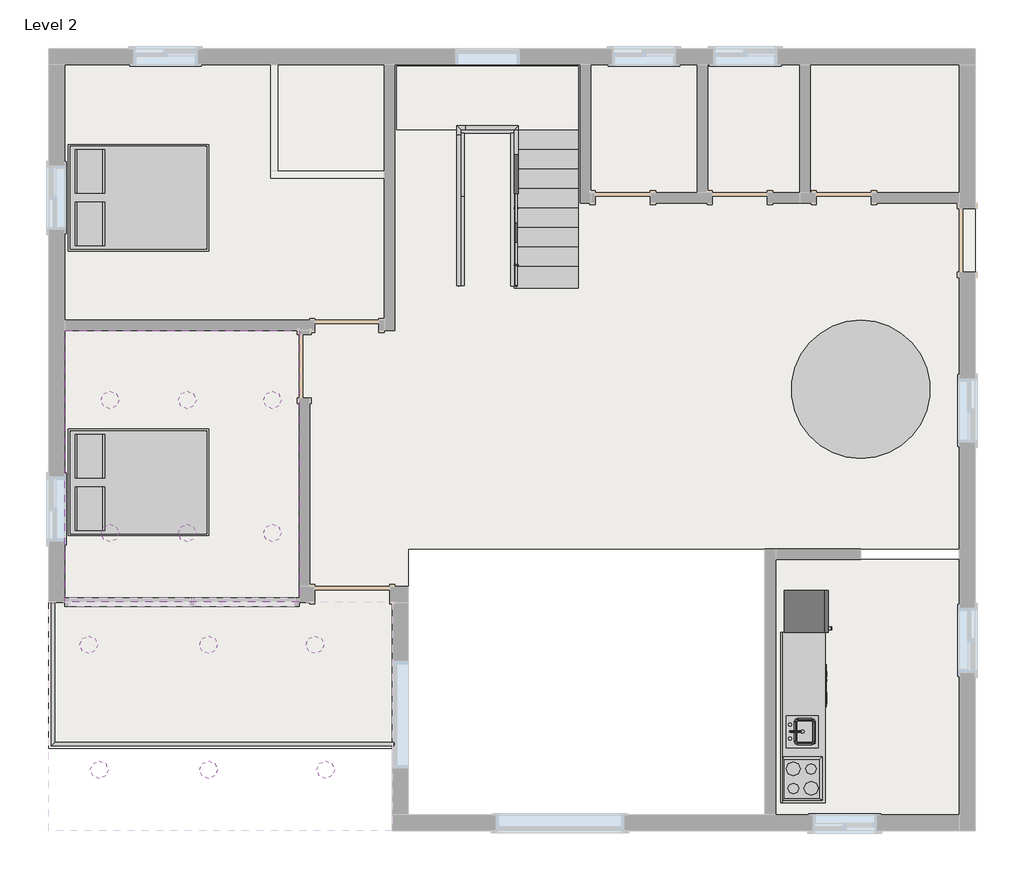
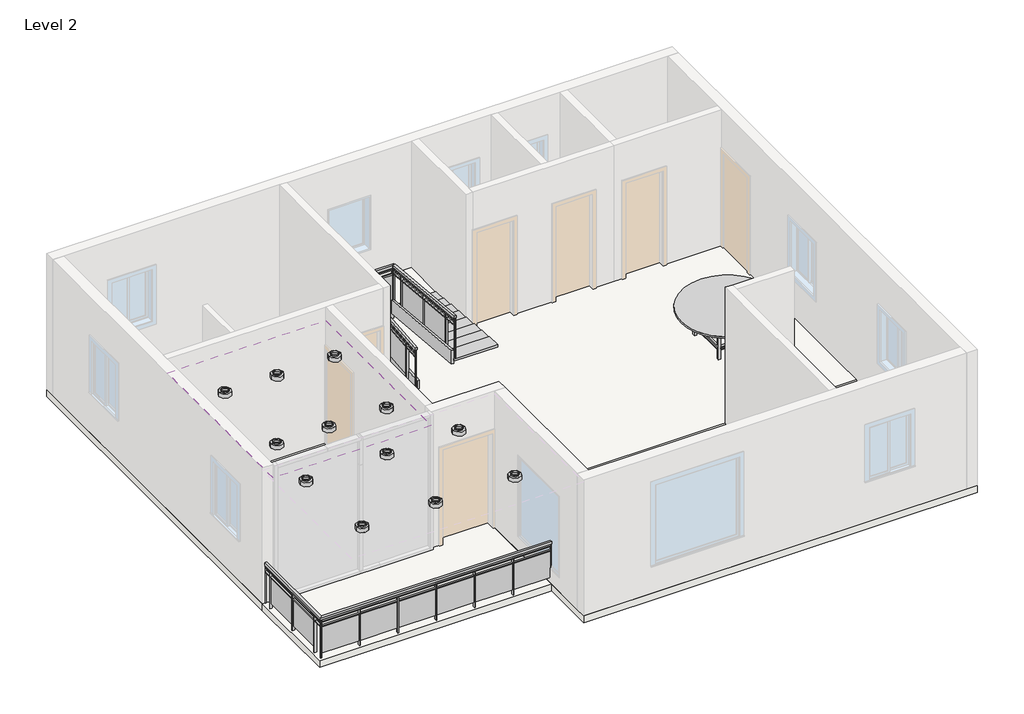
# One storey, part 2 of 2: 12 light fixtures, 4 furniture elements, 4 proxies, 3 members, 3 slabs, 2 railings, 1 covering, 1 flow terminal, 1 stair flight.
"""IFC4 building model written with IfcOpenShell, lengths in millimetres."""

from ifc_helpers import new_model, si_unit, frame, origin, place, context, project, spatial, polyline, outline, extrude, faceted_brep, transform, mapped, element, save
from components import proxy_a6faaae8, proxy_45b28599, kitchenette_medium_kitchenette_medium_844211aa, proxy_c523a7b7, flow_terminal_871c2e40, furniture_1d2926bd, furniture_8d292e24, furniture_7cf74a4d, ceiling_light_flat_round_100w_277v_0a96185f, non_monolithic_landing_fd591c5a, stair_flight_cd86263c

model = new_model("IFC4")

# Units and contexts
model_context = context("Model", 3, world=origin())
ifc_project = project(units=[si_unit("LENGTHUNIT", "METRE", prefix="MILLI")], contexts=[model_context])

# Site, building, storey
site = spatial("IfcSite", under=ifc_project)
building = spatial("IfcBuilding", under=site)
storey = spatial("IfcBuildingStorey", under=building, Name="Level 2", Elevation=3200.4)

# Proxies
placement = place(None, origin())
proxy_shape = proxy_a6faaae8(model_context)
element("IfcBuildingElementProxy", 1, Name="Cook Top-4 Unit2 : 22\" x 20\"", ObjectType="Cook Top-4 Unit2 : 22\" x 20\"", at=placement, inside=storey, context=model_context, shape_type="MappedRepresentation", body=[
    mapped(proxy_shape, transform((-1644.6867944, 4013.4230289, 3200.4), x_axis=(0.0, 1.0000000000000009, 0.0), y_axis=(-1.0000000000000009, 0.0, 0.0), z_axis=(0.0, 0.0, 1.0))),
])
proxy_2_shape = proxy_45b28599(model_context)
element("IfcBuildingElementProxy", 2, Name="Dishwasher : 24\" x 24\" x 34\"", ObjectType="Dishwasher : 24\" x 24\" x 34\"", at=placement, inside=storey, context=model_context, shape_type="MappedRepresentation", body=[
    mapped(proxy_2_shape, transform((-1352.8372296, 4964.6055604, 3200.4), x_axis=(0.0, 1.0000000000000009, 0.0), y_axis=(-1.0000000000000009, 0.0, 0.0), z_axis=(0.0, 0.0, 1.0))),
])
kitchenette_medium_kitchenette_medium_shape = kitchenette_medium_kitchenette_medium_844211aa(model_context)
element("IfcBuildingElementProxy", 3, Name="Kitchenette - Medium : Kitchenette - Medium", ObjectType="Kitchenette - Medium : Kitchenette - Medium", at=placement, inside=storey, context=model_context, shape_type="MappedRepresentation", body=[
    mapped(kitchenette_medium_kitchenette_medium_shape, transform((-1949.4867944, 4337.585324, 3200.4), x_axis=(0.0, 1.0000000000000009, 0.0), y_axis=(-1.0000000000000009, 0.0, 0.0), z_axis=(0.0, 0.0, 1.0))),
])
proxy_3_shape = proxy_c523a7b7(model_context)
element("IfcBuildingElementProxy", 4, Name="Refrigerator : 24\" x 25\" LH", ObjectType="Refrigerator : 24\" x 25\" LH", at=placement, inside=storey, context=model_context, shape_type="MappedRepresentation", body=[
    mapped(proxy_3_shape, transform((-1599.0378229, 6407.3730289, 3200.4), x_axis=(0.0, 1.0000000000000009, 0.0), y_axis=(-1.0000000000000009, 0.0, 0.0), z_axis=(0.0, 0.0, 1.0))),
])

# Covering
element("IfcCovering", 5, ObjectType="2' x 4' ACT System", at=placement, inside=storey, context=model_context, shape_type="SweptSolid", body=[
    extrude(outline(polyline([(-8845.5867944, 6540.7230289), (-12198.3867944, 6540.7230289), (-12198.3867944, 10426.9230289), (-8845.5867944, 10426.9230289), (-8845.5867944, 6540.7230289)])), frame((0.0, 0.0, 5943.6), z_axis=(0.0, 0.0, 1.0), x_axis=(1.0, 0.0, 0.0)), (0.0, 0.0, 1.0), 57.15),
])

# Flow terminal
flow_terminal_shape = flow_terminal_871c2e40(model_context)
element("IfcFlowTerminal", 6, ObjectType="Sink Kitchen-Island : 18\" x 18\"", at=placement, inside=storey, context=model_context, shape_type="MappedRepresentation", body=[
    mapped(flow_terminal_shape, transform((-1642.3413933, 4670.8337884, 3186.0), x_axis=(0.0, 1.0000000000000009, 0.0), y_axis=(-1.0000000000000009, 0.0, 0.0), z_axis=(0.0, 0.0, 1.0))),
])

# Furniture
furniture_shape = furniture_1d2926bd(model_context)
element("IfcFurniture", 7, ObjectType="Bed-Box : Queen 60\" x 79\"", at=placement, inside=storey, context=model_context, shape_type="MappedRepresentation", body=[
    mapped(furniture_shape, transform((-11378.7163026, 7916.0705699, 3200.4), x_axis=(0.0, 1.0000000000000002, 0.0), y_axis=(-1.0000000000000002, 0.0, 0.0), z_axis=(0.0, 0.0, 1.0))),
])
element("IfcFurniture", 8, ObjectType="Bed-Box : Queen 60\" x 79\"", at=placement, inside=storey, context=model_context, shape_type="MappedRepresentation", body=[
    mapped(furniture_shape, transform((-11378.7163026, 11992.7705699, 3200.4), x_axis=(0.0, 1.0000000000000002, 0.0), y_axis=(-1.0000000000000002, 0.0, 0.0), z_axis=(0.0, 0.0, 1.0))),
])
furniture_2_shape = furniture_8d292e24(model_context)
element("IfcFurniture", 9, ObjectType="Counter Top w Sink Hole : 24\" Depth", at=placement, inside=storey, context=model_context, shape_type="MappedRepresentation", body=[
    mapped(furniture_2_shape, transform((-1949.4867944, 4870.985324, 3186.0), x_axis=(0.0, 1.0000000000000009, 0.0), y_axis=(-1.0000000000000009, 0.0, 0.0), z_axis=(0.0, 0.0, 1.0))),
])
furniture_3_shape = furniture_7cf74a4d(model_context)
element("IfcFurniture", 10, ObjectType="Table-Dining Round w Chairs : 60\" Diameter", at=placement, inside=storey, context=model_context, shape_type="MappedRepresentation", body=[
    mapped(furniture_3_shape, transform((-910.1687616, 9773.6017175, 3200.4), x_axis=(1.0, 0.0, 0.0), y_axis=(0.0, 1.0, 0.0), z_axis=(0.0, 0.0, 1.0))),
])

# Light fixtures
ceiling_light_flat_round_100w_277v_shape = ceiling_light_flat_round_100w_277v_0a96185f(model_context)
element("IfcLightFixture", 11, ObjectType="Ceiling Light - Flat Round : 100W - 277V", at=placement, inside=storey, context=model_context, shape_type="MappedRepresentation", body=[
    mapped(ceiling_light_flat_round_100w_277v_shape, transform((-11855.4867944, 5931.1230289, 3759.2), x_axis=(1.0, 0.0, 0.0), y_axis=(0.0, 1.0, 0.0), z_axis=(0.0, 0.0, 1.0))),
])
element("IfcLightFixture", 12, ObjectType="Ceiling Light - Flat Round : 100W - 277V", at=placement, inside=storey, context=model_context, shape_type="MappedRepresentation", body=[
    mapped(ceiling_light_flat_round_100w_277v_shape, transform((-10140.9867944, 5931.1230289, 3759.2), x_axis=(1.0, 0.0, 0.0), y_axis=(0.0, 1.0, 0.0), z_axis=(0.0, 0.0, 1.0))),
])
element("IfcLightFixture", 13, ObjectType="Ceiling Light - Flat Round : 100W - 277V", at=placement, inside=storey, context=model_context, shape_type="MappedRepresentation", body=[
    mapped(ceiling_light_flat_round_100w_277v_shape, transform((-8616.9867944, 5931.1230289, 3759.2), x_axis=(1.0, 0.0, 0.0), y_axis=(0.0, 1.0, 0.0), z_axis=(0.0, 0.0, 1.0))),
])
element("IfcLightFixture", 14, ObjectType="Ceiling Light - Flat Round : 100W - 277V", at=placement, inside=storey, context=model_context, shape_type="MappedRepresentation", body=[
    mapped(ceiling_light_flat_round_100w_277v_shape, transform((-8464.5867944, 4140.4230289, 3759.2), x_axis=(1.0, 0.0, 0.0), y_axis=(0.0, 1.0, 0.0), z_axis=(0.0, 0.0, 1.0))),
])
element("IfcLightFixture", 15, ObjectType="Ceiling Light - Flat Round : 100W - 277V", at=placement, inside=storey, context=model_context, shape_type="MappedRepresentation", body=[
    mapped(ceiling_light_flat_round_100w_277v_shape, transform((-10140.9867944, 4140.4230289, 3759.2), x_axis=(1.0, 0.0, 0.0), y_axis=(0.0, 1.0, 0.0), z_axis=(0.0, 0.0, 1.0))),
])
element("IfcLightFixture", 16, ObjectType="Ceiling Light - Flat Round : 100W - 277V", at=placement, inside=storey, context=model_context, shape_type="MappedRepresentation", body=[
    mapped(ceiling_light_flat_round_100w_277v_shape, transform((-11703.0867944, 4140.4230289, 3759.2), x_axis=(1.0, 0.0, 0.0), y_axis=(0.0, 1.0, 0.0), z_axis=(0.0, 0.0, 1.0))),
])
element("IfcLightFixture", 17, ObjectType="Ceiling Light - Flat Round : 100W - 277V", at=placement, inside=storey, context=model_context, shape_type="MappedRepresentation", body=[
    mapped(ceiling_light_flat_round_100w_277v_shape, transform((-11550.6867944, 9436.3230289, 3505.2), x_axis=(1.0, 0.0, 0.0), y_axis=(0.0, 1.0, 0.0), z_axis=(0.0, 0.0, 1.0))),
])
element("IfcLightFixture", 18, ObjectType="Ceiling Light - Flat Round : 100W - 277V", at=placement, inside=storey, context=model_context, shape_type="MappedRepresentation", body=[
    mapped(ceiling_light_flat_round_100w_277v_shape, transform((-10445.7867944, 9436.3230289, 3505.2), x_axis=(1.0, 0.0, 0.0), y_axis=(0.0, 1.0, 0.0), z_axis=(0.0, 0.0, 1.0))),
])
element("IfcLightFixture", 19, ObjectType="Ceiling Light - Flat Round : 100W - 277V", at=placement, inside=storey, context=model_context, shape_type="MappedRepresentation", body=[
    mapped(ceiling_light_flat_round_100w_277v_shape, transform((-9226.5867944, 9436.3230289, 3505.2), x_axis=(1.0, 0.0, 0.0), y_axis=(0.0, 1.0, 0.0), z_axis=(0.0, 0.0, 1.0))),
])
element("IfcLightFixture", 20, ObjectType="Ceiling Light - Flat Round : 100W - 277V", at=placement, inside=storey, context=model_context, shape_type="MappedRepresentation", body=[
    mapped(ceiling_light_flat_round_100w_277v_shape, transform((-11550.6867944, 7531.3230289, 3505.2), x_axis=(1.0, 0.0, 0.0), y_axis=(0.0, 1.0, 0.0), z_axis=(0.0, 0.0, 1.0))),
])
element("IfcLightFixture", 21, ObjectType="Ceiling Light - Flat Round : 100W - 277V", at=placement, inside=storey, context=model_context, shape_type="MappedRepresentation", body=[
    mapped(ceiling_light_flat_round_100w_277v_shape, transform((-10445.7867944, 7531.3230289, 3505.2), x_axis=(1.0, 0.0, 0.0), y_axis=(0.0, 1.0, 0.0), z_axis=(0.0, 0.0, 1.0))),
])
element("IfcLightFixture", 22, ObjectType="Ceiling Light - Flat Round : 100W - 277V", at=placement, inside=storey, context=model_context, shape_type="MappedRepresentation", body=[
    mapped(ceiling_light_flat_round_100w_277v_shape, transform((-9226.5867944, 7531.3230289, 3505.2), x_axis=(1.0, 0.0, 0.0), y_axis=(0.0, 1.0, 0.0), z_axis=(0.0, 0.0, 1.0))),
])

# Members
element("IfcMember", 23, ObjectType="Stringer - 2\" Width", at=placement, inside=storey, context=model_context, shape_type="SweptSolid", body=[
    extrude(outline(polyline([(11074.6230289, 3200.4), (11074.6230289, 3389.0086921), (12352.7274155, 3505.2), (13259.0230289, 3505.2), (13259.0230289, 3281.5335978), (12366.5534535, 3200.4), (11074.6230289, 3200.4)])), frame((-6534.1867944, 0.0, 0.0), z_axis=(1.0, 0.0, 0.0), x_axis=(0.0, 1.0, 0.0)), (0.0, 0.0, 1.0), 50.8),
])
element("IfcMember", 24, ObjectType="Stringer - 2\" Width", at=placement, inside=storey, context=model_context, shape_type="SweptSolid", body=[
    extrude(outline(polyline([(13259.0230289, 3621.3376891), (13259.0230289, 3315.2807765), (11064.8419954, 3514.7517796), (11064.8419954, 3820.8086921), (13259.0230289, 3621.3376891)])), frame((-5812.9737939, 0.0, 0.0), z_axis=(1.0, 0.0, 0.0), x_axis=(0.0, 1.0, 0.0)), (0.0, 0.0, 1.0), 50.8),
])
element("IfcMember", 25, ObjectType="Stringer - 2\" Width", at=placement, inside=storey, context=model_context, shape_type="SweptSolid", body=[
    extrude(outline(polyline([(-6534.1867944, 13309.8230289), (-5762.1737939, 13309.8230289), (-5762.1737939, 13259.0230289), (-6534.1867944, 13259.0230289), (-6534.1867944, 13309.8230289)])), frame((0.0, 0.0, 3200.4), z_axis=(0.0, 0.0, 1.0), x_axis=(1.0, 0.0, 0.0)), (0.0, 0.0, 1.0), 304.8),
])

# Railings
element("IfcRailing", 26, ObjectType="Glass Panel - Bottom Fill", at=placement, inside=storey, context=model_context, shape_type="SolidModel", body=[
    faceted_brep([(-6584.9867944, 11074.6230289, 4140.2), (-6584.9867944, 11074.6230289, 4089.1905146), (-6534.1867944, 11074.6230289, 4089.1905146), (-6534.1867944, 11074.6230289, 4140.2), (-6534.1867944, 13284.4230289, 4290.0814237), (-6534.1867944, 13233.6230289, 4336.4727273), (-6584.9867944, 13233.6230289, 4336.4727273), (-6457.9867944, 13309.8230289, 4343.4), (-6457.9867944, 13309.8230289, 4292.6), (-5762.1737939, 13309.8230289, 4292.6), (-5762.1737939, 13309.8230289, 4343.4), (-6457.9867944, 13360.6230289, 4343.4), (-5711.3737939, 13360.6230289, 4343.4), (-6584.9867944, 13284.4230289, 4290.0814237), (-6584.9867944, 13233.6230289, 4343.4), (-6584.9867944, 13284.4230289, 4292.6), (-6534.1867944, 13284.4230289, 4292.6), (-6534.1867944, 13233.6230289, 4343.4), (-6584.9867944, 13360.6230289, 4343.4), (-6584.9867944, 13360.6230289, 4292.6), (-6534.1867944, 13309.8230289, 4292.6), (-6534.1867944, 13309.8230289, 4343.4), (-6457.9867944, 13360.6230289, 4292.6), (-5711.3737939, 13360.6230289, 4292.6), (-5711.3737939, 13300.0419954, 4343.4), (-5762.1737939, 13300.0419954, 4343.4), (-5762.1737939, 13297.7376557, 4292.6), (-5711.3737939, 13297.7376557, 4292.6)], [[[0, 1, 2, 3]], [[3, 2, 4, 5]], [[0, 3, 5, 6]], [[7, 8, 9, 10]], [[11, 7, 10, 12]], [[1, 0, 6, 13]], [[2, 1, 13, 4]], [[13, 6, 14, 15]], [[4, 13, 15, 16]], [[5, 4, 16, 17]], [[6, 5, 17, 14]], [[15, 14, 18, 19]], [[16, 15, 19, 20]], [[17, 16, 20, 21]], [[14, 17, 21, 18]], [[19, 18, 11, 22]], [[20, 19, 22, 8]], [[21, 20, 8, 7]], [[18, 21, 7, 11]], [[22, 11, 12, 23]], [[8, 22, 23, 9]], [[24, 25, 26, 27]], [[23, 12, 24, 27]], [[9, 23, 27, 26]], [[10, 9, 26, 25]], [[12, 10, 25, 24]]]),
    faceted_brep([(-5711.3737939, 13300.0419954, 4368.8), (-5711.3737939, 13297.7376557, 4318.0), (-5762.1737939, 13297.7376557, 4318.0), (-5762.1737939, 13300.0419954, 4368.8), (-5711.3737939, 11064.8419954, 4572.0), (-5762.1737939, 11064.8419954, 4572.0), (-5762.1737939, 11064.8419954, 4520.9905146), (-5711.3737939, 11064.8419954, 4520.9905146)], [[[0, 1, 2, 3]], [[4, 5, 6, 7]], [[3, 2, 6, 5]], [[0, 3, 5, 4]], [[1, 0, 4, 7]], [[2, 1, 7, 6]]]),
    faceted_brep([(-6546.8867944, 11074.6230289, 4051.3523714), (-6572.2867944, 11074.6230289, 4051.3523714), (-6572.2867944, 11074.6230289, 4025.8476286), (-6546.8867944, 11074.6230289, 4025.8476286), (-6546.8867944, 13321.4253812, 4255.6071307), (-6546.8867944, 13323.7249892, 4230.3114432), (-6572.2867944, 13349.0206766, 4232.6110512), (-6572.2867944, 13346.7210687, 4257.9067386)], [[[0, 1, 2, 3]], [[4, 5, 6, 7]], [[1, 0, 4, 7]], [[2, 1, 7, 6]], [[3, 2, 6, 5]], [[0, 3, 5, 4]]]),
    faceted_brep([(-6548.0887547, 13322.5230289, 4254.5), (-6573.3844421, 13347.9230289, 4254.5), (-6571.0848342, 13347.9230289, 4229.1), (-6545.7891467, 13322.5230289, 4229.1), (-5749.4737939, 13322.5230289, 4254.5), (-5749.4737939, 13322.5230289, 4229.1), (-5724.0737939, 13347.9230289, 4229.1), (-5724.0737939, 13347.9230289, 4254.5)], [[[0, 1, 2, 3]], [[4, 5, 6, 7]], [[1, 0, 4, 7]], [[2, 1, 7, 6]], [[3, 2, 6, 5]], [[0, 3, 5, 4]]]),
    faceted_brep([(-5749.4737939, 13300.6180803, 4279.9), (-5724.0737939, 13300.6180803, 4279.9), (-5724.0737939, 13299.4659105, 4254.5), (-5749.4737939, 13299.4659105, 4254.5), (-5749.4737939, 11064.8419954, 4483.1523714), (-5749.4737939, 11064.8419954, 4457.6476286), (-5724.0737939, 11064.8419954, 4457.6476286), (-5724.0737939, 11064.8419954, 4483.1523714)], [[[0, 1, 2, 3]], [[4, 5, 6, 7]], [[1, 0, 4, 7]], [[2, 1, 7, 6]], [[3, 2, 6, 5]], [[0, 3, 5, 4]]]),
    faceted_brep([(-6546.8867944, 11074.6230289, 3949.7523714), (-6572.2867944, 11074.6230289, 3949.7523714), (-6572.2867944, 11074.6230289, 3924.2476286), (-6546.8867944, 11074.6230289, 3924.2476286), (-6546.8867944, 13321.4253812, 4154.0071307), (-6546.8867944, 13323.7249892, 4128.7114432), (-6572.2867944, 13349.0206766, 4131.0110512), (-6572.2867944, 13346.7210687, 4156.3067386)], [[[0, 1, 2, 3]], [[4, 5, 6, 7]], [[1, 0, 4, 7]], [[2, 1, 7, 6]], [[3, 2, 6, 5]], [[0, 3, 5, 4]]]),
    faceted_brep([(-6548.0887547, 13322.5230289, 4152.9), (-6573.3844421, 13347.9230289, 4152.9), (-6571.0848342, 13347.9230289, 4127.5), (-6545.7891467, 13322.5230289, 4127.5), (-5749.4737939, 13322.5230289, 4152.9), (-5749.4737939, 13322.5230289, 4127.5), (-5724.0737939, 13347.9230289, 4127.5), (-5724.0737939, 13347.9230289, 4152.9)], [[[0, 1, 2, 3]], [[4, 5, 6, 7]], [[1, 0, 4, 7]], [[2, 1, 7, 6]], [[3, 2, 6, 5]], [[0, 3, 5, 4]]]),
    faceted_brep([(-5749.4737939, 13300.6180803, 4178.3), (-5724.0737939, 13300.6180803, 4178.3), (-5724.0737939, 13299.4659105, 4152.9), (-5749.4737939, 13299.4659105, 4152.9), (-5749.4737939, 11064.8419954, 4381.5523714), (-5749.4737939, 11064.8419954, 4356.0476286), (-5724.0737939, 11064.8419954, 4356.0476286), (-5724.0737939, 11064.8419954, 4381.5523714)], [[[0, 1, 2, 3]], [[4, 5, 6, 7]], [[1, 0, 4, 7]], [[2, 1, 7, 6]], [[3, 2, 6, 5]], [[0, 3, 5, 4]]]),
    faceted_brep([(-5749.4737939, 13322.5230289, 4254.5), (-5724.0737939, 13347.9230289, 4254.5), (-5724.0737939, 13347.9230289, 4229.1), (-5749.4737939, 13322.5230289, 4229.1), (-5749.4737939, 13300.6180803, 4254.5), (-5749.4737939, 13299.4659105, 4229.1), (-5724.0737939, 13299.4659105, 4229.1), (-5724.0737939, 13300.6180803, 4254.5)], [[[0, 1, 2, 3]], [[4, 5, 6, 7]], [[1, 0, 4, 7]], [[2, 1, 7, 6]], [[3, 2, 6, 5]], [[0, 3, 5, 4]]]),
    faceted_brep([(-5749.4737939, 13322.5230289, 4152.9), (-5724.0737939, 13347.9230289, 4152.9), (-5724.0737939, 13347.9230289, 4127.5), (-5749.4737939, 13322.5230289, 4127.5), (-5749.4737939, 13300.6180803, 4152.9), (-5749.4737939, 13299.4659105, 4127.5), (-5724.0737939, 13299.4659105, 4127.5), (-5724.0737939, 13300.6180803, 4152.9)], [[[0, 1, 2, 3]], [[4, 5, 6, 7]], [[1, 0, 4, 7]], [[2, 1, 7, 6]], [[3, 2, 6, 5]], [[0, 3, 5, 4]]]),
    extrude(outline(polyline([(11363.2919954, 4430.5158105), (11375.9919954, 4429.361265), (11375.9919954, 3606.8), (11363.2919954, 3606.8), (11363.2919954, 4430.5158105)])), frame((-5762.1737939, 0.0, 0.0), z_axis=(1.0, 0.0, 0.0), x_axis=(0.0, 1.0, 0.0)), (0.0, 0.0, 1.0), 50.8),
    extrude(outline(polyline([(12182.4419954, 3646.0545455), (11369.6419954, 3719.9454545), (11369.6419954, 4328.3385377), (12182.4419954, 4254.4476286), (12182.4419954, 3646.0545455)])), frame((-5736.5886369, 0.0, 0.0), z_axis=(1.0, 0.0, 0.0), x_axis=(0.0, 1.0, 0.0)), (0.0, 0.0, 1.0), 6.35),
    extrude(outline(polyline([(12176.0919954, 4356.6249014), (12188.7919954, 4355.4703559), (12188.7919954, 3556.0), (12176.0919954, 3556.0), (12176.0919954, 4356.6249014)])), frame((-5762.1737939, 0.0, 0.0), z_axis=(1.0, 0.0, 0.0), x_axis=(0.0, 1.0, 0.0)), (0.0, 0.0, 1.0), 50.8),
    extrude(outline(polyline([(12995.2419954, 3569.8545455), (12182.4419954, 3643.7454545), (12182.4419954, 4254.4476286), (12995.2419954, 4180.5567196), (12995.2419954, 3569.8545455)])), frame((-5736.5886369, 0.0, 0.0), z_axis=(1.0, 0.0, 0.0), x_axis=(0.0, 1.0, 0.0)), (0.0, 0.0, 1.0), 6.35),
    extrude(outline(polyline([(12988.8919954, 4282.7339923), (13001.5919954, 4281.5794468), (13001.5919954, 3479.8), (12988.8919954, 3479.8), (12988.8919954, 4282.7339923)])), frame((-5762.1737939, 0.0, 0.0), z_axis=(1.0, 0.0, 0.0), x_axis=(0.0, 1.0, 0.0)), (0.0, 0.0, 1.0), 50.8),
    extrude(outline(polyline([(-5748.1302942, 13309.8230289), (-5748.1302942, 13360.6230289), (-5735.4302942, 13360.6230289), (-5735.4302942, 13309.8230289), (-5748.1302942, 13309.8230289)])), frame((0.0, 0.0, 3429.0), z_axis=(0.0, 0.0, 1.0), x_axis=(1.0, 0.0, 0.0)), (0.0, 0.0, 1.0), 800.1),
    extrude(outline(polyline([(-6554.5802942, 13341.7581859), (-5741.7802942, 13341.7581859), (-5741.7802942, 13335.4081859), (-6554.5802942, 13335.4081859), (-6554.5802942, 13341.7581859)])), frame((0.0, 0.0, 3530.6), z_axis=(0.0, 0.0, 1.0), x_axis=(1.0, 0.0, 0.0)), (0.0, 0.0, 1.0), 596.9),
    extrude(outline(polyline([(-6560.9302942, 13309.8230289), (-6560.9302942, 13360.6230289), (-6548.2302942, 13360.6230289), (-6548.2302942, 13309.8230289), (-6560.9302942, 13309.8230289)])), frame((0.0, 0.0, 3429.0), z_axis=(0.0, 0.0, 1.0), x_axis=(1.0, 0.0, 0.0)), (0.0, 0.0, 1.0), 800.1),
    extrude(outline(polyline([(13011.3730289, 4201.9158105), (13024.0730289, 4203.0703559), (13024.0730289, 3378.2), (13011.3730289, 3378.2), (13011.3730289, 4201.9158105)])), frame((-6584.9867944, 0.0, 0.0), z_axis=(1.0, 0.0, 0.0), x_axis=(0.0, 1.0, 0.0)), (0.0, 0.0, 1.0), 50.8),
    extrude(outline(polyline([(12204.9230289, 3417.4545455), (12204.9230289, 4027.0021741), (13017.7230289, 4100.8930832), (13017.7230289, 3491.3454545), (12204.9230289, 3417.4545455)])), frame((-6566.1219514, 0.0, 0.0), z_axis=(1.0, 0.0, 0.0), x_axis=(0.0, 1.0, 0.0)), (0.0, 0.0, 1.0), 6.35),
    extrude(outline(polyline([(12198.5730289, 4128.0249014), (12211.2730289, 4129.1794468), (12211.2730289, 3327.4), (12198.5730289, 3327.4), (12198.5730289, 4128.0249014)])), frame((-6584.9867944, 0.0, 0.0), z_axis=(1.0, 0.0, 0.0), x_axis=(0.0, 1.0, 0.0)), (0.0, 0.0, 1.0), 50.8),
    extrude(outline(polyline([(11392.1230289, 3341.2545455), (11392.1230289, 3953.111265), (12204.9230289, 4027.0021741), (12204.9230289, 3415.1454545), (11392.1230289, 3341.2545455)])), frame((-6566.1219514, 0.0, 0.0), z_axis=(1.0, 0.0, 0.0), x_axis=(0.0, 1.0, 0.0)), (0.0, 0.0, 1.0), 6.35),
    extrude(outline(polyline([(11385.7730289, 4054.1339923), (11398.4730289, 4055.2885377), (11398.4730289, 3251.2), (11385.7730289, 3251.2), (11385.7730289, 4054.1339923)])), frame((-6584.9867944, 0.0, 0.0), z_axis=(1.0, 0.0, 0.0), x_axis=(0.0, 1.0, 0.0)), (0.0, 0.0, 1.0), 50.8),
    extrude(outline(polyline([(13290.5169954, 4318.6564237), (13309.5669954, 4316.9246055), (13309.5669954, 3454.4), (13290.5169954, 3454.4), (13290.5169954, 4318.6564237)])), frame((-5746.2987939, 0.0, 0.0), z_axis=(1.0, 0.0, 0.0), x_axis=(0.0, 1.0, 0.0)), (0.0, 0.0, 1.0), 19.05),
    extrude(outline(polyline([(-5746.2987939, 13325.6980289), (-5746.2987939, 13344.7480289), (-5727.2487939, 13344.7480289), (-5727.2487939, 13325.6980289), (-5746.2987939, 13325.6980289)])), frame((0.0, 0.0, 3429.0), z_axis=(0.0, 0.0, 1.0), x_axis=(1.0, 0.0, 0.0)), (0.0, 0.0, 1.0), 863.6),
    extrude(outline(polyline([(-6550.0617944, 13325.6980289), (-6569.1117944, 13325.6980289), (-6569.1117944, 13344.7480289), (-6550.0617944, 13344.7480289), (-6550.0617944, 13325.6980289)])), frame((0.0, 0.0, 3429.0), z_axis=(0.0, 0.0, 1.0), x_axis=(1.0, 0.0, 0.0)), (0.0, 0.0, 1.0), 863.6),
    extrude(outline(polyline([(11058.4919954, 4521.5677873), (11077.5419954, 4519.8359691), (11077.5419954, 3632.2), (11058.4919954, 3632.2), (11058.4919954, 4521.5677873)])), frame((-5746.2987939, 0.0, 0.0), z_axis=(1.0, 0.0, 0.0), x_axis=(0.0, 1.0, 0.0)), (0.0, 0.0, 1.0), 19.05),
    extrude(outline(polyline([(11068.2730289, 4088.6132418), (11087.3230289, 4090.34506), (11087.3230289, 3225.8), (11068.2730289, 3225.8), (11068.2730289, 4088.6132418)])), frame((-6569.1117944, 0.0, 0.0), z_axis=(1.0, 0.0, 0.0), x_axis=(0.0, 1.0, 0.0)), (0.0, 0.0, 1.0), 19.05),
])
element("IfcRailing", 27, ObjectType="Glass Panel - Bottom Fill", at=placement, inside=storey, context=model_context, shape_type="SolidModel", body=[
    faceted_brep([(-12338.0867944, 6540.7230289, 4114.8), (-12338.0867944, 6540.7230289, 4064.0), (-12388.8867944, 6540.7230289, 4064.0), (-12388.8867944, 6540.7230289, 4114.8), (-12338.0867944, 4534.1230289, 4114.8), (-12338.0867944, 4534.1230289, 4064.0), (-12388.8867944, 4483.3230289, 4064.0), (-12388.8867944, 4483.3230289, 4114.8), (-7486.6867944, 4534.1230289, 4114.8), (-7486.6867944, 4483.3230289, 4114.8), (-7486.6867944, 4483.3230289, 4064.0), (-7486.6867944, 4534.1230289, 4064.0)], [[[0, 1, 2, 3]], [[1, 0, 4, 5]], [[2, 1, 5, 6]], [[3, 2, 6, 7]], [[0, 3, 7, 4]], [[8, 9, 10, 11]], [[5, 4, 8, 11]], [[6, 5, 11, 10]], [[7, 6, 10, 9]], [[4, 7, 9, 8]]]),
    faceted_brep([(-12376.1867944, 6540.7230289, 4025.9), (-12350.7867944, 6540.7230289, 4025.9), (-12350.7867944, 6540.7230289, 4000.5), (-12376.1867944, 6540.7230289, 4000.5), (-12376.1867944, 4496.0230289, 4025.9), (-12350.7867944, 4521.4230289, 4025.9), (-12350.7867944, 4521.4230289, 4000.5), (-12376.1867944, 4496.0230289, 4000.5), (-7486.6867944, 4496.0230289, 4025.9), (-7486.6867944, 4496.0230289, 4000.5), (-7486.6867944, 4521.4230289, 4000.5), (-7486.6867944, 4521.4230289, 4025.9)], [[[0, 1, 2, 3]], [[1, 0, 4, 5]], [[2, 1, 5, 6]], [[3, 2, 6, 7]], [[0, 3, 7, 4]], [[8, 9, 10, 11]], [[5, 4, 8, 11]], [[6, 5, 11, 10]], [[7, 6, 10, 9]], [[4, 7, 9, 8]]]),
    faceted_brep([(-12376.1867944, 6540.7230289, 3924.3), (-12350.7867944, 6540.7230289, 3924.3), (-12350.7867944, 6540.7230289, 3898.9), (-12376.1867944, 6540.7230289, 3898.9), (-12376.1867944, 4496.0230289, 3924.3), (-12350.7867944, 4521.4230289, 3924.3), (-12350.7867944, 4521.4230289, 3898.9), (-12376.1867944, 4496.0230289, 3898.9), (-7486.6867944, 4496.0230289, 3924.3), (-7486.6867944, 4496.0230289, 3898.9), (-7486.6867944, 4521.4230289, 3898.9), (-7486.6867944, 4521.4230289, 3924.3)], [[[0, 1, 2, 3]], [[1, 0, 4, 5]], [[2, 1, 5, 6]], [[3, 2, 6, 7]], [[0, 3, 7, 4]], [[8, 9, 10, 11]], [[5, 4, 8, 11]], [[6, 5, 11, 10]], [[7, 6, 10, 9]], [[4, 7, 9, 8]]]),
    extrude(outline(polyline([(-8299.4867944, 4515.2581859), (-7486.6867944, 4515.2581859), (-7486.6867944, 4508.9081859), (-8299.4867944, 4508.9081859), (-8299.4867944, 4515.2581859)])), frame((0.0, 0.0, 3302.0), z_axis=(0.0, 0.0, 1.0), x_axis=(1.0, 0.0, 0.0)), (0.0, 0.0, 1.0), 596.9),
    extrude(outline(polyline([(-8305.8367944, 4483.3230289), (-8305.8367944, 4534.1230289), (-8293.1367944, 4534.1230289), (-8293.1367944, 4483.3230289), (-8305.8367944, 4483.3230289)])), frame((0.0, 0.0, 3200.4), z_axis=(0.0, 0.0, 1.0), x_axis=(1.0, 0.0, 0.0)), (0.0, 0.0, 1.0), 800.1),
    extrude(outline(polyline([(-9112.2867944, 4515.2581859), (-8299.4867944, 4515.2581859), (-8299.4867944, 4508.9081859), (-9112.2867944, 4508.9081859), (-9112.2867944, 4515.2581859)])), frame((0.0, 0.0, 3302.0), z_axis=(0.0, 0.0, 1.0), x_axis=(1.0, 0.0, 0.0)), (0.0, 0.0, 1.0), 596.9),
    extrude(outline(polyline([(-9118.6367944, 4483.3230289), (-9118.6367944, 4534.1230289), (-9105.9367944, 4534.1230289), (-9105.9367944, 4483.3230289), (-9118.6367944, 4483.3230289)])), frame((0.0, 0.0, 3200.4), z_axis=(0.0, 0.0, 1.0), x_axis=(1.0, 0.0, 0.0)), (0.0, 0.0, 1.0), 800.1),
    extrude(outline(polyline([(-9925.0867944, 4515.2581859), (-9112.2867944, 4515.2581859), (-9112.2867944, 4508.9081859), (-9925.0867944, 4508.9081859), (-9925.0867944, 4515.2581859)])), frame((0.0, 0.0, 3302.0), z_axis=(0.0, 0.0, 1.0), x_axis=(1.0, 0.0, 0.0)), (0.0, 0.0, 1.0), 596.9),
    extrude(outline(polyline([(-9931.4367944, 4483.3230289), (-9931.4367944, 4534.1230289), (-9918.7367944, 4534.1230289), (-9918.7367944, 4483.3230289), (-9931.4367944, 4483.3230289)])), frame((0.0, 0.0, 3200.4), z_axis=(0.0, 0.0, 1.0), x_axis=(1.0, 0.0, 0.0)), (0.0, 0.0, 1.0), 800.1),
    extrude(outline(polyline([(-10737.8867944, 4515.2581859), (-9925.0867944, 4515.2581859), (-9925.0867944, 4508.9081859), (-10737.8867944, 4508.9081859), (-10737.8867944, 4515.2581859)])), frame((0.0, 0.0, 3302.0), z_axis=(0.0, 0.0, 1.0), x_axis=(1.0, 0.0, 0.0)), (0.0, 0.0, 1.0), 596.9),
    extrude(outline(polyline([(-10744.2367944, 4483.3230289), (-10744.2367944, 4534.1230289), (-10731.5367944, 4534.1230289), (-10731.5367944, 4483.3230289), (-10744.2367944, 4483.3230289)])), frame((0.0, 0.0, 3200.4), z_axis=(0.0, 0.0, 1.0), x_axis=(1.0, 0.0, 0.0)), (0.0, 0.0, 1.0), 800.1),
    extrude(outline(polyline([(-11550.6867944, 4515.2581859), (-10737.8867944, 4515.2581859), (-10737.8867944, 4508.9081859), (-11550.6867944, 4508.9081859), (-11550.6867944, 4515.2581859)])), frame((0.0, 0.0, 3302.0), z_axis=(0.0, 0.0, 1.0), x_axis=(1.0, 0.0, 0.0)), (0.0, 0.0, 1.0), 596.9),
    extrude(outline(polyline([(-11557.0367944, 4483.3230289), (-11557.0367944, 4534.1230289), (-11544.3367944, 4534.1230289), (-11544.3367944, 4483.3230289), (-11557.0367944, 4483.3230289)])), frame((0.0, 0.0, 3200.4), z_axis=(0.0, 0.0, 1.0), x_axis=(1.0, 0.0, 0.0)), (0.0, 0.0, 1.0), 800.1),
    extrude(outline(polyline([(-12363.4867944, 4515.2581859), (-11550.6867944, 4515.2581859), (-11550.6867944, 4508.9081859), (-12363.4867944, 4508.9081859), (-12363.4867944, 4515.2581859)])), frame((0.0, 0.0, 3302.0), z_axis=(0.0, 0.0, 1.0), x_axis=(1.0, 0.0, 0.0)), (0.0, 0.0, 1.0), 596.9),
    extrude(outline(polyline([(-12388.8867944, 4718.2730289), (-12338.0867944, 4718.2730289), (-12338.0867944, 4705.5730289), (-12388.8867944, 4705.5730289), (-12388.8867944, 4718.2730289)])), frame((0.0, 0.0, 3200.4), z_axis=(0.0, 0.0, 1.0), x_axis=(1.0, 0.0, 0.0)), (0.0, 0.0, 1.0), 800.1),
    extrude(outline(polyline([(-12356.9516374, 5524.7230289), (-12356.9516374, 4711.9230289), (-12363.3016374, 4711.9230289), (-12363.3016374, 5524.7230289), (-12356.9516374, 5524.7230289)])), frame((0.0, 0.0, 3302.0), z_axis=(0.0, 0.0, 1.0), x_axis=(1.0, 0.0, 0.0)), (0.0, 0.0, 1.0), 596.9),
    extrude(outline(polyline([(-12388.8867944, 5531.0730289), (-12338.0867944, 5531.0730289), (-12338.0867944, 5518.3730289), (-12388.8867944, 5518.3730289), (-12388.8867944, 5531.0730289)])), frame((0.0, 0.0, 3200.4), z_axis=(0.0, 0.0, 1.0), x_axis=(1.0, 0.0, 0.0)), (0.0, 0.0, 1.0), 800.1),
    extrude(outline(polyline([(-12356.9516374, 6337.5230289), (-12356.9516374, 5524.7230289), (-12363.3016374, 5524.7230289), (-12363.3016374, 6337.5230289), (-12356.9516374, 6337.5230289)])), frame((0.0, 0.0, 3302.0), z_axis=(0.0, 0.0, 1.0), x_axis=(1.0, 0.0, 0.0)), (0.0, 0.0, 1.0), 596.9),
    extrude(outline(polyline([(-12388.8867944, 6343.8730289), (-12338.0867944, 6343.8730289), (-12338.0867944, 6331.1730289), (-12388.8867944, 6331.1730289), (-12388.8867944, 6343.8730289)])), frame((0.0, 0.0, 3200.4), z_axis=(0.0, 0.0, 1.0), x_axis=(1.0, 0.0, 0.0)), (0.0, 0.0, 1.0), 800.1),
    extrude(outline(polyline([(-12373.0117944, 4518.2480289), (-12353.9617944, 4518.2480289), (-12353.9617944, 4499.1980289), (-12373.0117944, 4499.1980289), (-12373.0117944, 4518.2480289)])), frame((0.0, 0.0, 3200.4), z_axis=(0.0, 0.0, 1.0), x_axis=(1.0, 0.0, 0.0)), (0.0, 0.0, 1.0), 863.6),
    extrude(outline(polyline([(-7499.3867944, 4499.1980289), (-7499.3867944, 4518.2480289), (-7480.3367944, 4518.2480289), (-7480.3367944, 4499.1980289), (-7499.3867944, 4499.1980289)])), frame((0.0, 0.0, 3200.4), z_axis=(0.0, 0.0, 1.0), x_axis=(1.0, 0.0, 0.0)), (0.0, 0.0, 1.0), 863.6),
    extrude(outline(polyline([(-12373.0117944, 6547.0730289), (-12353.9617944, 6547.0730289), (-12353.9617944, 6528.0230289), (-12373.0117944, 6528.0230289), (-12373.0117944, 6547.0730289)])), frame((0.0, 0.0, 3200.4), z_axis=(0.0, 0.0, 1.0), x_axis=(1.0, 0.0, 0.0)), (0.0, 0.0, 1.0), 863.6),
])

# Slabs
element("IfcSlab", 28, ObjectType="6\"", at=placement, inside=storey, context=model_context, shape_type="SweptSolid", body=[
    extrude(outline(polyline([(831.8132056, 14465.5230289), (831.8132056, 7302.7230289), (-7283.4867944, 7302.7230289), (-7283.4867944, 4445.2230289), (-7512.0867944, 4445.2230289), (-12426.9867944, 4445.2230289), (-12426.9867944, 6540.7230289), (-12426.9867944, 14465.5230289), (831.8132056, 14465.5230289)])), frame((0.0, 0.0, 3048.0), z_axis=(0.0, 0.0, 1.0), x_axis=(1.0, 0.0, 0.0)), (0.0, 0.0, 1.0), 152.4),
])
element("IfcSlab", 29, ObjectType="6\"", at=placement, inside=storey, context=model_context, shape_type="SweptSolid", body=[
    extrude(outline(polyline([(-7512.0867944, 3264.1230289), (-7512.0867944, 6540.7230289), (-7283.4867944, 6540.7230289), (-7283.4867944, 3492.7230289), (-2178.0867944, 3492.7230289), (-2178.0867944, 7150.3230289), (831.8132056, 7150.3230289), (831.8132056, 3264.1230289), (-7512.0867944, 3264.1230289)])), frame((0.0, 0.0, 3048.0), z_axis=(0.0, 0.0, 1.0), x_axis=(1.0, 0.0, 0.0)), (0.0, 0.0, 1.0), 152.4),
])
non_monolithic_landing_shape = non_monolithic_landing_fd591c5a(model_context)
element("IfcSlab", 30, ObjectType="Non-Monolithic Landing", at=placement, inside=storey, context=model_context, shape_type="MappedRepresentation", body=[
    mapped(non_monolithic_landing_shape, transform((0.0, 0.0, 0.0), x_axis=(1.0, 0.0, 0.0), y_axis=(0.0, 1.0, 0.0), z_axis=(0.0, 0.0, 1.0))),
])

# Stair flight
stair_flight_shape = stair_flight_cd86263c(model_context)
element("IfcStairFlight", 31, ObjectType="2\" Tread 1\" Nosing 1/4\" Riser", at=placement, inside=storey, context=model_context, shape_type="MappedRepresentation", body=[
    mapped(stair_flight_shape, transform((0.0, 0.0, 0.0), x_axis=(1.0, 0.0, 0.0), y_axis=(0.0, 1.0, 0.0), z_axis=(0.0, 0.0, 1.0))),
])

save(model, "model.ifc")

# Revit data of these elements
# Type "Cook Top-4 Unit2 : 22\" x 20\""
#   Depth = 1' - 8"
#   Width = 1' - 10"
#   Burner Material = Steel, Chrome Plated
#   Cooktop Material = Steel, Polished
#   Default Elevation = 0
#   Assembly Code = ""
# Type "Dishwasher : 24\" x 24\" x 34\""
#   Label = "DW"
#   Assembly Code = "E1090400"
#   Depth = 2' - 0"
#   Height = 2' - 10"
#   Width = 2' - 0"
#   Dishwasher Material = Steel, Paint Finish, Ivory, Glossy
#   Panel Face Material = Plastic, Opaque Black
#   Default Elevation = 0
# Type "Kitchenette - Medium : Kitchenette - Medium"
#   Assembly Code = "E1090400"
#   Counter Length = 8' - 0"
#   Cabinet Width = 4' - 6"
#   Cabinet Height = 2' - 10 1/2"
#   Cabinet Depth = 2' - 0"
#   Toe Depth = 0' - 3"
#   Toe Height = 0' - 3 1/2"
#   Cabinet Material = Cabinets
#   Door/Drawer Material = Cabinets
#   Handle Material = Cabinets - Handles
#   Default Elevation = 0
# Type "Refrigerator : 24\" x 25\" LH"
#   Label = "REF."
#   Assembly Code = "E1090400"
#   Depth = 2' - 0 3/4"
#   Handle = 0' - 1 1/2"
#   Height = 5' - 3 1/2"
#   Rear Clearance = 0' - 2"
#   Top Door Height = 1' - 8"
#   Width = 1' - 11 1/2"
#   Material = Steel, Paint Finish, Ivory, Glossy
#   Default Elevation = 0
# Type "2' x 4' ACT System"
#   Assembly Code = "C3030210"
#   built-in parameter 1002203 = 1 (stored number, unit not read)
#   built-in parameter 1002202 = 1 (stored number, unit not read)
#   Layers, outside or top first: 0' - 1 5/8" "Default" (function 1); 0' - 0 5/8" "Softwood, Lumber" (function 5)
# Type "Sink Kitchen-Island : 18\" x 18\""
#   Assembly Code = "D2010410"
#   Counter Height = 3' - 0"
#   Depth = 1' - 6"
#   Width = 1' - 6"
#   Faucet Material = Steel, Polished
#   Sink Material = Steel, Polished
#   Default Elevation = 0
# Type "Bed-Box : Queen 60\" x 79\""
#   Assembly Code = "E2020200"
#   Length = 6' - 7"
#   Width = 5' - 0"
#   Frame Material = Birch
#   Mattress Material = Linen, White
#   Default Elevation = 0
# Type "Counter Top w Sink Hole : 24\" Depth"
#   Assembly Code = "C1030400"
#   Counter Thickness = 0' - 1 1/2"
#   Depth = 2' - 1"
#   Height = 3' - 0"
#   Length [instance default] = 8' - 0"
#   Sink Location [instance default] = 2' - 0"
#   Sink Location To Wall [instance default] = 0' - 6"
#   Sink Opening Depth [instance default] = 1' - 3"
#   Sink Opening Width [instance default] = 2' - 3"
#   Counter Top Material = none
#   Default Elevation = 0
# Type "Table-Dining Round w Chairs : 60\" Diameter"
#   Assembly Code = "E2020200"
#   Radius = 3' - 3"
#   Diameter = 6' - 6"
#   Height = 2' - 6"
#   Chairs = 10
#   Base Material = Pine
#   Top Material = Laminate, Linen, Matte
#   Default Elevation = 0
# Type "Ceiling Light - Flat Round : 100W - 277V"
#   Lamp = "A-19"
#   Assembly Code = "D5020220"
#   Wattage = 100 W
#   built-in parameter 1150110 = 1 (stored number, unit not read)
#   built-in parameter 1114217 = 1 (stored number, unit not read)
#   built-in parameter 1150109 = 1 (stored number, unit not read)
#   built-in parameter 1150113 = 1 (stored number, unit not read)
#   built-in parameter 1150115 = 1 (stored number, unit not read)
#   built-in parameter 1150105 = 557.042 (stored number, unit not read)
#   Light Source Symbol Size = 2' - 0"
#   built-in parameter 1150112 = 1 (stored number, unit not read)
#   built-in parameter 1150114 = 1 (stored number, unit not read)
#   built-in parameter 1150107 = 2800 (stored number, unit not read)
#   built-in parameter 1150106 = 5.57042 (stored number, unit not read)
#   Emit from Circle Diameter = 0' - 10"
#   built-in parameter 1150104 = 1.6258 (stored number, unit not read)
#   Ballast Voltage = 277 V
#   built-in parameter 1114218 = 1 (stored number, unit not read)
#   built-in parameter 1150133 = 10 (stored number, unit not read)
#   Lumens = 1750 lm
#   Apparent Load = 100 VA
#   built-in parameter 1150134 = 4
#   built-in parameter 1150137 = 1
#   Color Filter = 16777215
#   built-in parameter 1140040 [instance default] = 1
#   Ballast Number of Poles = 1
#   Light Box Material = Steel, Paint Finish, Dark Gray, Matte
#   Diffuser Material = Glass, White, High Luminance
#   Wattage Comments = ""
#   Emit Shape Visible in Rendering = no
#   Dimming Lamp Color Temperature Shift = (empty or 0)
#   Default Elevation = 0
# Type "Glass Panel - Bottom Fill"
#   Assembly Code = "C2010400"
#   built-in parameter 1008612 = 0.0416667 (stored number, unit not read)
#   built-in parameter 1008611 = 0.0416667 (stored number, unit not read)
#   built-in parameter 1008609 = 0.333333 (stored number, unit not read)
#   built-in parameter 1008604 = 0.166667 (stored number, unit not read)
#   built-in parameter 1008603 = 0.166667 (stored number, unit not read)
#   Railing Height = 3' - 0"
#   built-in parameter 1008632 = 1
#   built-in parameter 1008631 = 1
#   built-in parameter 1008630 = 1
#   built-in parameter 1008610 = 2
#   built-in parameter 1008618 = Baluster - Square : 3/4"
# Type "6\""
#   Assembly Code = "B1010"
#   Function = 0
#   Layers, outside or top first: 0' - 6" "flooring" (function 1)
# Element 1 (IfcBuildingElementProxy, "Cook Top-4 Unit2 : 22\" x 20\"")
#   Phase Created = New Construction
#   Materials on its faces: "Steel, Chrome Plated", "Steel, Polished"
# Element 2 (IfcBuildingElementProxy, "Dishwasher : 24\" x 24\" x 34\"")
#   Phase Created = New Construction
#   Materials on its faces: "Steel, Paint Finish, Ivory, Glossy", "Plastic, Opaque Black"
# Element 3 (IfcBuildingElementProxy, "Kitchenette - Medium : Kitchenette - Medium")
#   Phase Created = New Construction
#   Materials on its faces: "Cabinets", "Cabinets - Handles"
# Element 4 (IfcBuildingElementProxy, "Refrigerator : 24\" x 25\" LH")
#   Phase Created = New Construction
#   Materials on its faces: "Steel, Paint Finish, Ivory, Glossy", "Steel, Chrome Plated"
# Element 5 (IfcCovering, "2' x 4' ACT System")
#   Height Offset From Level = 9' - 0"
#   Phase Created = New Construction
#   Materials on its faces: "Softwood, Lumber", "Default"
# Element 6 (IfcFlowTerminal, "Sink Kitchen-Island : 18\" x 18\"")
#   Mark = "6"
#   Phase Created = New Construction
#   Materials on its faces: "Steel, Polished"
# Elements 7, 8 (IfcFurniture, "Bed-Box : Queen 60\" x 79\"")
#   Phase Created = New Construction
#   Materials on its faces: "Birch", "Linen, White"
# Element 9 (IfcFurniture, "Counter Top w Sink Hole : 24\" Depth")
#   Sink Opening Depth = 1' - 2"
#   Sink Location To Wall = 0' - 6"
#   Length = 8' - 0"
#   Sink Location = 3' - 4"
#   Sink Opening Width = 1' - 4"
#   Phase Created = New Construction
#   Materials on its faces: "Counter Top"
# Element 10 (IfcFurniture, "Table-Dining Round w Chairs : 60\" Diameter")
#   Phase Created = New Construction
#   Materials on its faces: "Pine", "Laminate, Linen, Matte"
# Element 11 (IfcLightFixture, "Ceiling Light - Flat Round : 100W - 277V")
#   Mark = "7"
#   built-in parameter 1140040 = 1
#   Phase Created = New Construction
#   Materials on its faces: "Glass, White, High Luminance", "Steel, Paint Finish, Dark Gray, Matte"
# Element 12 (IfcLightFixture, "Ceiling Light - Flat Round : 100W - 277V")
#   Mark = "8"
#   built-in parameter 1140040 = 1
#   Phase Created = New Construction
#   Materials on its faces: "Glass, White, High Luminance", "Steel, Paint Finish, Dark Gray, Matte"
# Element 13 (IfcLightFixture, "Ceiling Light - Flat Round : 100W - 277V")
#   Mark = "9"
#   built-in parameter 1140040 = 1
#   Phase Created = New Construction
#   Materials on its faces: "Glass, White, High Luminance", "Steel, Paint Finish, Dark Gray, Matte"
# Element 14 (IfcLightFixture, "Ceiling Light - Flat Round : 100W - 277V")
#   Mark = "10"
#   built-in parameter 1140040 = 1
#   Phase Created = New Construction
#   Materials on its faces: "Glass, White, High Luminance", "Steel, Paint Finish, Dark Gray, Matte"
# Element 15 (IfcLightFixture, "Ceiling Light - Flat Round : 100W - 277V")
#   Mark = "11"
#   built-in parameter 1140040 = 1
#   Phase Created = New Construction
#   Materials on its faces: "Glass, White, High Luminance", "Steel, Paint Finish, Dark Gray, Matte"
# Element 16 (IfcLightFixture, "Ceiling Light - Flat Round : 100W - 277V")
#   Mark = "12"
#   built-in parameter 1140040 = 1
#   Phase Created = New Construction
#   Materials on its faces: "Glass, White, High Luminance", "Steel, Paint Finish, Dark Gray, Matte"
# Element 17 (IfcLightFixture, "Ceiling Light - Flat Round : 100W - 277V")
#   Mark = "13"
#   built-in parameter 1140040 = 1
#   Phase Created = New Construction
#   Materials on its faces: "Glass, White, High Luminance", "Steel, Paint Finish, Dark Gray, Matte"
# Element 18 (IfcLightFixture, "Ceiling Light - Flat Round : 100W - 277V")
#   Mark = "14"
#   built-in parameter 1140040 = 1
#   Phase Created = New Construction
#   Materials on its faces: "Glass, White, High Luminance", "Steel, Paint Finish, Dark Gray, Matte"
# Element 19 (IfcLightFixture, "Ceiling Light - Flat Round : 100W - 277V")
#   Mark = "15"
#   built-in parameter 1140040 = 1
#   Phase Created = New Construction
#   Materials on its faces: "Glass, White, High Luminance", "Steel, Paint Finish, Dark Gray, Matte"
# Element 20 (IfcLightFixture, "Ceiling Light - Flat Round : 100W - 277V")
#   Mark = "16"
#   built-in parameter 1140040 = 1
#   Phase Created = New Construction
#   Materials on its faces: "Glass, White, High Luminance", "Steel, Paint Finish, Dark Gray, Matte"
# Element 21 (IfcLightFixture, "Ceiling Light - Flat Round : 100W - 277V")
#   Mark = "17"
#   built-in parameter 1140040 = 1
#   Phase Created = New Construction
#   Materials on its faces: "Glass, White, High Luminance", "Steel, Paint Finish, Dark Gray, Matte"
# Element 22 (IfcLightFixture, "Ceiling Light - Flat Round : 100W - 277V")
#   Mark = "18"
#   built-in parameter 1140040 = 1
#   Phase Created = New Construction
#   Materials on its faces: "Glass, White, High Luminance", "Steel, Paint Finish, Dark Gray, Matte"
# Elements 23, 24, 25 (IfcMember, "Stringer - 2\" Width")
#   Phase Created = New Construction
# Elements 26, 27 (IfcRailing, "Glass Panel - Bottom Fill")
#   Phase Created = New Construction
#   Materials on its faces: "Glass"
# Element 28 (IfcSlab, "6\"")
#   Height Offset From Level = 0' - 0"
#   Phase Created = New Construction
#   Materials on its faces: "flooring"
# Element 29 (IfcSlab, "6\"")
#   built-in parameter 1001955 = -1.5708 (stored number, unit not read)
#   Height Offset From Level = 0' - 0"
#   Phase Created = New Construction
#   Materials on its faces: "flooring"
# Element 30 (IfcSlab, "Non-Monolithic Landing")
#   Phase Created = New Construction
# Element 31 (IfcStairFlight, "2\" Tread 1\" Nosing 1/4\" Riser")
#   Phase Created = New Construction
# Materials
#   "Steel, Chrome Plated": class "Metal", colour RGB 17 17 17, transparency 0, Description = "Chromiuim plated steel", Cost = 0
#   "Steel, Polished": class "Metal", colour RGB 57 57 57, transparency 0, Description = "Polished steel", Cost = 0
#   "Steel, Paint Finish, Ivory, Glossy": class "Metal", colour RGB 247 247 239, transparency 0, Description = "Steel, paint finish, ivory, glossy", Cost = 0
#   "Plastic, Opaque Black": class "Plastic", colour RGB 0 0 0, transparency 0.7, Description = "Plastic, generic, opaque black", Cost = 0
#   "Cabinets": colour RGB 249 249 249, transparency 0
#   "Cabinets - Handles": class "Metal", colour RGB 57 57 57, transparency 0
#   "Default": colour RGB 127 127 127, transparency 0
#   "Softwood, Lumber": class "Wood", colour RGB 144 112 60, transparency 0, Description = "Pinus Echinata", Cost = 0
#   "Birch": class "Wood", colour RGB 224 178 126, transparency 0, Description = "Betula Alleghaniensis", Cost = 0
#   "Linen, White": class "Textile", colour RGB 247 247 239, transparency 0, Description = "Linen, white", Cost = 0
#   "Pine": class "Wood", colour RGB 223 192 134, transparency 0, Description = "Pinus Echinata", Cost = 0
#   "Laminate, Linen, Matte": class "Plastic", colour RGB 249 239 230, transparency 0, Description = "Plastic Laminate - Linen, Matte", Cost = 0
#   "Steel, Paint Finish, Dark Gray, Matte": class "Metal", colour RGB 98 98 98, transparency 0, Description = "Steel, paint finish, dark gray, matte", Cost = 0
#   "Glass, White, High Luminance": class "Glass", colour RGB 249 250 249, transparency 0.8, Description = "physical material", Cost = 0
#   "flooring": class "Generic", colour RGB 120 120 120, transparency 0, Cost = 0
#   "Counter Top": class "Wood", colour RGB 226 177 128, transparency 0
#   "Glass": class "Glass", colour RGB 0 128 192, transparency 0.75, Description = "Soda Lime Glass", Cost = 0
